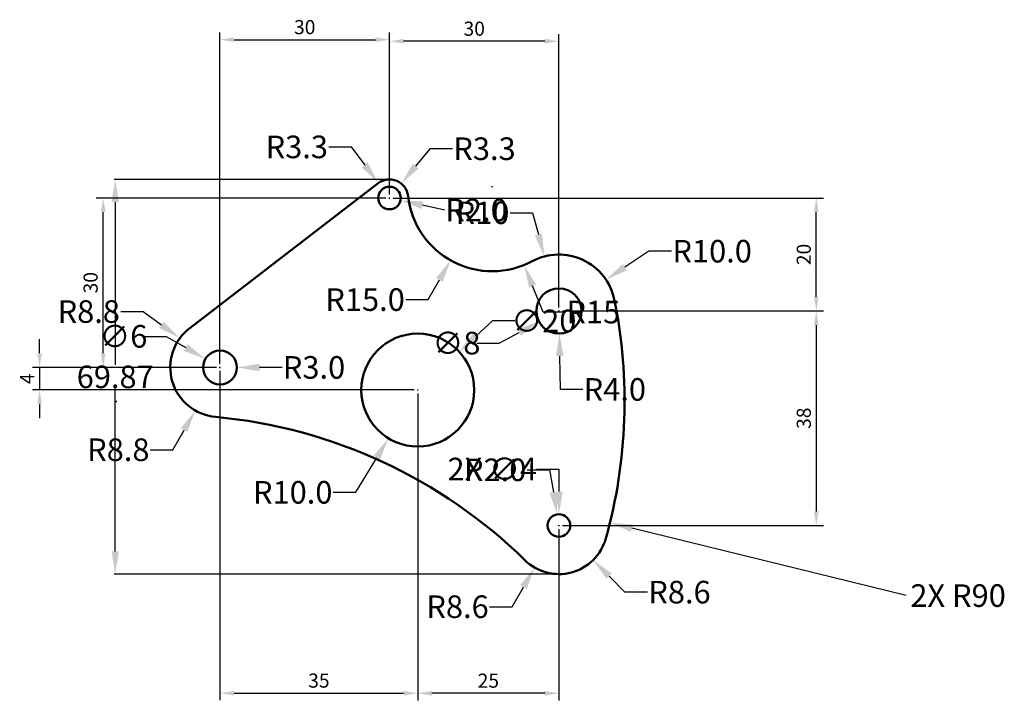
# Model space of a CAD drawing. Units: millimetres. Extents: x 257 to 432, y 502 to 622.
import ezdxf

# ---------------------------------------------------------------- set-up
doc = ezdxf.new("R2010")
doc.units = ezdxf.units.MM
doc.layers.add('M-DIMS', color=2, linetype='Continuous', lineweight=25)
doc.layers.add('M-OUTL', color=7, linetype='Continuous', lineweight=50)
doc.styles.get("Standard").update_dxf_attribs({"font": 'arial.ttf'})
doc.dimstyles.new('ISO-25', dxfattribs={"dimtxt": 2.5, "dimasz": 2.5, "dimexe": 1.25, "dimexo": 0.625, "dimtad": 1, "dimtxsty": 'Standard', "dimcen": 2.5, "dimadec": 0, "dimazin": 0, "dimtfac": 1, "dimtmove": 0, "dimatfit": 3, "dimfxl": 1, "dimarcsym": 0})
doc.dimstyles.get("Standard").update_dxf_attribs({"dimtxt": 4, "dimasz": 4, "dimexe": 0.18, "dimexo": 0.0625, "dimgap": 0.09, "dimtad": 0, "dimtih": 1, "dimtoh": 1, "dimdec": 1, "dimzin": 0, "dimdsep": 46, "dimtxsty": 'Standard', "dimcen": 0.09, "dimadec": 0, "dimazin": 0, "dimtfac": 1, "dimtdec": 1, "dimtofl": 0, "dimtmove": 0, "dimatfit": 3, "dimfxl": 1, "dimtolj": 1, "dimtzin": 0, "dimarcsym": 0})

# ---------------------------------------------------------------- blocks, each defined once
blk = doc.blocks.new('*D1')
at = {"layer": 'Defpoints', "color": 0, "transparency": 16777216}
for p in [(292.89, 560.64), (260.95, 556.64), (327.89, 556.64)]:
    blk.add_point(p, dxfattribs=at)
at = {"layer": 'M-DIMS', "color": 0, "lineweight": -2, "transparency": 16777216}
for p, q in [((260.95, 563.14), (260.95, 565.64)), ((292.27, 560.64), (259.7, 560.64)), ((260.95, 560.64), (260.95, 556.64)), ((327.27, 556.64), (259.7, 556.64)), ((260.95, 554.14), (260.95, 551.64))]:
    blk.add_line(p, q, dxfattribs=at)
at = {"layer": 'M-DIMS', "color": 0, "transparency": 16777216}
for points in [[(260.53, 563.14), (261.36, 563.14), (260.95, 560.64)], [(260.53, 554.14), (261.36, 554.14), (260.95, 556.64)]]:
    blk.add_solid(points, dxfattribs=at)
at = {"layer": 'M-DIMS', "color": 0, "transparency": 16777216, "insert": (259.07, 558.64), "char_height": 2.5, "attachment_point": 5, "rotation": 90}
blk.add_mtext('4', dxfattribs=at)
blk = doc.blocks.new('*D2')
at = {"layer": 'Defpoints', "color": 0, "transparency": 16777216}
for p in [(322.89, 618.4), (322.89, 590.64), (352.89, 570.64)]:
    blk.add_point(p, dxfattribs=at)
at = {"layer": 'M-DIMS', "color": 0, "lineweight": -2, "transparency": 16777216}
for p, q in [((322.89, 591.26), (322.89, 619.65)), ((352.89, 571.26), (352.89, 619.65)), ((350.39, 618.4), (325.39, 618.4))]:
    blk.add_line(p, q, dxfattribs=at)
at = {"layer": 'M-DIMS', "color": 0, "transparency": 16777216}
for points in [[(325.39, 618.82), (325.39, 617.99), (322.89, 618.4)], [(350.39, 618.82), (350.39, 617.99), (352.89, 618.4)]]:
    blk.add_solid(points, dxfattribs=at)
at = {"layer": 'M-DIMS', "color": 0, "transparency": 16777216, "insert": (337.89, 620.3), "char_height": 2.5, "attachment_point": 5}
blk.add_mtext('30', dxfattribs=at)
blk = doc.blocks.new('*D3')
at = {"layer": 'Defpoints', "color": 0, "transparency": 16777216}
for p in [(322.89, 618.68), (322.89, 590.64), (292.89, 560.64)]:
    blk.add_point(p, dxfattribs=at)
at = {"layer": 'M-DIMS', "color": 0, "lineweight": -2, "transparency": 16777216}
for p, q in [((292.89, 561.26), (292.89, 619.93)), ((322.89, 591.26), (322.89, 619.93)), ((295.39, 618.68), (320.39, 618.68))]:
    blk.add_line(p, q, dxfattribs=at)
at = {"layer": 'M-DIMS', "color": 0, "transparency": 16777216}
for points in [[(295.39, 619.09), (295.39, 618.26), (292.89, 618.68)], [(320.39, 619.09), (320.39, 618.26), (322.89, 618.68)]]:
    blk.add_solid(points, dxfattribs=at)
at = {"layer": 'M-DIMS', "color": 0, "transparency": 16777216, "insert": (307.89, 620.58), "char_height": 2.5, "attachment_point": 5}
blk.add_mtext('30', dxfattribs=at)
blk = doc.blocks.new('*D4')
at = {"layer": 'Defpoints', "color": 0, "transparency": 16777216}
for p in [(327.89, 556.64), (352.89, 532.64), (327.89, 502.93)]:
    blk.add_point(p, dxfattribs=at)
at = {"layer": 'M-DIMS', "color": 0, "lineweight": -2, "transparency": 16777216}
for p, q in [((327.89, 556.01), (327.89, 501.68)), ((352.89, 532.01), (352.89, 501.68)), ((350.39, 502.93), (330.39, 502.93))]:
    blk.add_line(p, q, dxfattribs=at)
at = {"layer": 'M-DIMS', "color": 0, "transparency": 16777216}
for points in [[(330.39, 503.35), (330.39, 502.52), (327.89, 502.93)], [(350.39, 503.35), (350.39, 502.52), (352.89, 502.93)]]:
    blk.add_solid(points, dxfattribs=at)
at = {"layer": 'M-DIMS', "color": 0, "transparency": 16777216, "insert": (340.39, 504.84), "char_height": 2.5, "attachment_point": 5}
blk.add_mtext('25', dxfattribs=at)
blk = doc.blocks.new('*D5')
at = {"layer": 'Defpoints', "color": 0, "transparency": 16777216}
for p in [(352.89, 570.64), (352.89, 532.64), (398.45, 532.64)]:
    blk.add_point(p, dxfattribs=at)
at = {"layer": 'M-DIMS', "color": 0, "lineweight": -2, "transparency": 16777216}
for p, q in [((353.52, 570.64), (399.7, 570.64)), ((398.45, 568.14), (398.45, 535.14)), ((353.52, 532.64), (399.7, 532.64))]:
    blk.add_line(p, q, dxfattribs=at)
at = {"layer": 'M-DIMS', "color": 0, "transparency": 16777216}
for points in [[(398.03, 568.14), (398.86, 568.14), (398.45, 570.64)], [(398.03, 535.14), (398.86, 535.14), (398.45, 532.64)]]:
    blk.add_solid(points, dxfattribs=at)
at = {"layer": 'M-DIMS', "color": 0, "transparency": 16777216, "insert": (396.55, 551.64), "char_height": 2.5, "attachment_point": 5, "rotation": 90}
blk.add_mtext('38', dxfattribs=at)
blk = doc.blocks.new('*D6')
at = {"layer": 'Defpoints', "color": 0, "transparency": 16777216}
for p in [(322.89, 590.64), (398.45, 590.64), (352.89, 570.64)]:
    blk.add_point(p, dxfattribs=at)
at = {"layer": 'M-DIMS', "color": 0, "lineweight": -2, "transparency": 16777216}
for p, q in [((323.52, 590.64), (399.7, 590.64)), ((398.45, 573.14), (398.45, 588.14)), ((353.52, 570.64), (399.7, 570.64))]:
    blk.add_line(p, q, dxfattribs=at)
at = {"layer": 'M-DIMS', "color": 0, "transparency": 16777216}
for points in [[(398.03, 588.14), (398.86, 588.14), (398.45, 590.64)], [(398.03, 573.14), (398.86, 573.14), (398.45, 570.64)]]:
    blk.add_solid(points, dxfattribs=at)
at = {"layer": 'M-DIMS', "color": 0, "transparency": 16777216, "insert": (396.55, 580.64), "char_height": 2.5, "attachment_point": 5, "rotation": 90}
blk.add_mtext('20', dxfattribs=at)
blk = doc.blocks.new('*D7')
at = {"layer": 'Defpoints', "color": 0, "transparency": 16777216}
for p in [(292.89, 560.64), (327.89, 556.64), (327.89, 502.94)]:
    blk.add_point(p, dxfattribs=at)
at = {"layer": 'M-DIMS', "color": 0, "lineweight": -2, "transparency": 16777216}
for p, q in [((292.89, 560.01), (292.89, 501.69)), ((327.89, 556.01), (327.89, 501.69)), ((295.39, 502.94), (325.39, 502.94))]:
    blk.add_line(p, q, dxfattribs=at)
at = {"layer": 'M-DIMS', "color": 0, "transparency": 16777216}
for points in [[(295.39, 503.36), (295.39, 502.53), (292.89, 502.94)], [(325.39, 503.36), (325.39, 502.53), (327.89, 502.94)]]:
    blk.add_solid(points, dxfattribs=at)
at = {"layer": 'M-DIMS', "color": 0, "transparency": 16777216, "insert": (310.39, 504.85), "char_height": 2.5, "attachment_point": 5}
blk.add_mtext('35', dxfattribs=at)
blk = doc.blocks.new('*D8')
at = {"layer": 'Defpoints', "color": 0, "transparency": 16777216}
for p in [(272.22, 590.64), (322.89, 590.64), (292.89, 560.64)]:
    blk.add_point(p, dxfattribs=at)
at = {"layer": 'M-DIMS', "color": 0, "lineweight": -2, "transparency": 16777216}
for p, q in [((322.27, 590.64), (270.97, 590.64)), ((272.22, 563.14), (272.22, 588.14)), ((292.27, 560.64), (270.97, 560.64))]:
    blk.add_line(p, q, dxfattribs=at)
at = {"layer": 'M-DIMS', "color": 0, "transparency": 16777216}
for points in [[(271.8, 588.14), (272.63, 588.14), (272.22, 590.64)], [(271.8, 563.14), (272.63, 563.14), (272.22, 560.64)]]:
    blk.add_solid(points, dxfattribs=at)
at = {"layer": 'M-DIMS', "color": 0, "transparency": 16777216, "insert": (270.31, 575.64), "char_height": 2.5, "attachment_point": 5, "rotation": 90}
blk.add_mtext('30', dxfattribs=at)
blk = doc.blocks.new('*D9')
at = {"layer": 'Defpoints', "color": 0, "transparency": 16777216}
for p in [(352.89, 532.64), (358.94, 526.53)]:
    blk.add_point(p, dxfattribs=at)
at = {"layer": 'M-DIMS', "color": 0, "lineweight": -2, "transparency": 16777216}
for p, q in [((352.8, 532.64), (352.98, 532.64)), ((352.89, 532.55), (352.89, 532.73)), ((364.57, 520.84), (361.76, 523.68)), ((368.57, 520.84), (364.57, 520.84))]:
    blk.add_line(p, q, dxfattribs=at)
at = {"layer": 'M-DIMS', "color": 0, "transparency": 16777216}
blk.add_solid([(362.23, 524.15), (361.28, 523.21), (358.94, 526.53)], dxfattribs=at)
at = {"layer": 'M-DIMS', "color": 0, "transparency": 16777216, "insert": (374.22, 520.84), "char_height": 4, "attachment_point": 5}
blk.add_mtext('\\A1;R8.6', dxfattribs=at)
blk = doc.blocks.new('*D10')
at = {"layer": 'Defpoints', "color": 0, "transparency": 16777216}
for p in [(361.22, 576.17), (352.89, 570.64)]:
    blk.add_point(p, dxfattribs=at)
at = {"layer": 'M-DIMS', "color": 0, "lineweight": -2, "transparency": 16777216}
for p, q in [((368.81, 581.22), (364.55, 578.39)), ((372.81, 581.22), (368.81, 581.22)), ((352.8, 570.64), (352.98, 570.64)), ((352.89, 570.55), (352.89, 570.73))]:
    blk.add_line(p, q, dxfattribs=at)
at = {"layer": 'M-DIMS', "color": 0, "transparency": 16777216}
blk.add_solid([(364.18, 578.94), (364.92, 577.83), (361.22, 576.17)], dxfattribs=at)
at = {"layer": 'M-DIMS', "color": 0, "transparency": 16777216, "insert": (380.01, 581.22), "char_height": 4, "attachment_point": 5}
blk.add_mtext('\\A1;R10.0', dxfattribs=at)
blk = doc.blocks.new('*D11')
at = {"layer": 'Defpoints', "color": 0, "transparency": 16777216}
for p in [(292.89, 560.64), (288.52, 553)]:
    blk.add_point(p, dxfattribs=at)
at = {"layer": 'M-DIMS', "color": 0, "lineweight": -2, "transparency": 16777216}
for p, q in [((292.8, 560.64), (292.98, 560.64)), ((292.89, 560.55), (292.89, 560.73)), ((284.54, 546.06), (286.53, 549.53)), ((280.54, 546.06), (284.54, 546.06))]:
    blk.add_line(p, q, dxfattribs=at)
at = {"layer": 'M-DIMS', "color": 0, "transparency": 16777216}
blk.add_solid([(285.95, 549.86), (287.11, 549.2), (288.52, 553)], dxfattribs=at)
at = {"layer": 'M-DIMS', "color": 0, "transparency": 16777216, "insert": (274.89, 546.06), "char_height": 4, "attachment_point": 5}
blk.add_mtext('\\A1;R8.8', dxfattribs=at)
blk = doc.blocks.new('*D12')
at = {"layer": 'Defpoints', "color": 0, "transparency": 16777216}
for p in [(324.98, 593.19), (322.89, 590.64)]:
    blk.add_point(p, dxfattribs=at)
at = {"layer": 'M-DIMS', "color": 0, "lineweight": -2, "transparency": 16777216}
for p, q in [((330.06, 599.37), (327.52, 596.28)), ((334.06, 599.37), (330.06, 599.37)), ((322.8, 590.64), (322.98, 590.64)), ((322.89, 590.55), (322.89, 590.73))]:
    blk.add_line(p, q, dxfattribs=at)
at = {"layer": 'M-DIMS', "color": 0, "transparency": 16777216}
blk.add_solid([(327.01, 596.7), (328.04, 595.85), (324.98, 593.19)], dxfattribs=at)
at = {"layer": 'M-DIMS', "color": 0, "transparency": 16777216, "insert": (339.71, 599.37), "char_height": 4, "attachment_point": 5}
blk.add_mtext('\\A1;R3.3', dxfattribs=at)
blk = doc.blocks.new('*D13')
at = {"layer": 'Defpoints', "color": 0, "transparency": 16777216}
for p in [(341.08, 592.67), (333.7, 579.61)]:
    blk.add_point(p, dxfattribs=at)
at = {"layer": 'M-DIMS', "color": 0, "lineweight": -2, "transparency": 16777216}
for p, q in [((340.99, 592.67), (341.17, 592.67)), ((341.08, 592.58), (341.08, 592.76)), ((329.76, 572.65), (331.73, 576.13)), ((325.76, 572.65), (329.76, 572.65))]:
    blk.add_line(p, q, dxfattribs=at)
at = {"layer": 'M-DIMS', "color": 0, "transparency": 16777216}
blk.add_solid([(331.15, 576.46), (332.31, 575.8), (333.7, 579.61)], dxfattribs=at)
at = {"layer": 'M-DIMS', "color": 0, "transparency": 16777216, "insert": (318.57, 572.65), "char_height": 4, "attachment_point": 5}
blk.add_mtext('\\A1;R15.0', dxfattribs=at)
blk = doc.blocks.new('*D14')
at = {"layer": 'Defpoints', "color": 0, "transparency": 16777216}
for p in [(322.89, 590.64), (324.84, 590.21)]:
    blk.add_point(p, dxfattribs=at)
at = {"layer": 'M-DIMS', "color": 0, "lineweight": -2, "transparency": 16777216}
for p, q in [((322.8, 590.64), (322.98, 590.64)), ((322.89, 590.55), (322.89, 590.73)), ((332.66, 588.51), (328.75, 589.36))]:
    blk.add_line(p, q, dxfattribs=at)
at = {"layer": 'M-DIMS', "color": 0, "transparency": 16777216}
blk.add_solid([(328.9, 590.01), (328.61, 588.71), (324.84, 590.21)], dxfattribs=at)
at = {"layer": 'M-DIMS', "color": 0, "transparency": 16777216, "insert": (338.3, 588.51), "char_height": 4, "attachment_point": 5}
blk.add_mtext('\\A1;R2.0', dxfattribs=at)
blk = doc.blocks.new('*D15')
at = {"layer": 'Defpoints', "color": 0, "transparency": 16777216}
for p in [(327.89, 556.64), (322.72, 548.08)]:
    blk.add_point(p, dxfattribs=at)
at = {"layer": 'M-DIMS', "color": 0, "lineweight": -2, "transparency": 16777216}
for p, q in [((327.8, 556.64), (327.98, 556.64)), ((327.89, 556.55), (327.89, 556.73)), ((316.95, 538.52), (320.65, 544.65)), ((312.95, 538.52), (316.95, 538.52))]:
    blk.add_line(p, q, dxfattribs=at)
at = {"layer": 'M-DIMS', "color": 0, "transparency": 16777216}
blk.add_solid([(320.08, 545), (321.22, 544.31), (322.72, 548.08)], dxfattribs=at)
at = {"layer": 'M-DIMS', "color": 0, "transparency": 16777216, "insert": (305.76, 538.52), "char_height": 4, "attachment_point": 5}
blk.add_mtext('\\A1;R10.0', dxfattribs=at)
blk = doc.blocks.new('*D16')
at = {"layer": 'Defpoints', "color": 0, "transparency": 16777216}
for p in [(352.56, 534.61), (352.89, 532.64)]:
    blk.add_point(p, dxfattribs=at)
at = {"layer": 'M-DIMS', "color": 0, "lineweight": -2, "transparency": 16777216}
for p, q in [((347.24, 542.5), (351.24, 542.5)), ((351.24, 542.5), (351.9, 538.55)), ((352.8, 532.64), (352.98, 532.64)), ((352.89, 532.55), (352.89, 532.73))]:
    blk.add_line(p, q, dxfattribs=at)
at = {"layer": 'M-DIMS', "color": 0, "transparency": 16777216}
blk.add_solid([(352.56, 538.66), (351.24, 538.44), (352.56, 534.61)], dxfattribs=at)
at = {"layer": 'M-DIMS', "color": 0, "transparency": 16777216, "insert": (341.6, 542.5), "char_height": 4, "attachment_point": 5}
blk.add_mtext('\\A1;R2.0', dxfattribs=at)
blk = doc.blocks.new('*D17')
at = {"layer": 'Defpoints', "color": 0, "transparency": 16777216}
for p in [(352.89, 570.64), (352.96, 566.64)]:
    blk.add_point(p, dxfattribs=at)
at = {"layer": 'M-DIMS', "color": 0, "lineweight": -2, "transparency": 16777216}
for p, q in [((352.8, 570.64), (352.98, 570.64)), ((352.89, 570.55), (352.89, 570.73)), ((353.14, 556.74), (353.04, 562.64)), ((357.14, 556.74), (353.14, 556.74))]:
    blk.add_line(p, q, dxfattribs=at)
at = {"layer": 'M-DIMS', "color": 0, "transparency": 16777216}
blk.add_solid([(353.7, 562.65), (352.37, 562.63), (352.96, 566.64)], dxfattribs=at)
at = {"layer": 'M-DIMS', "color": 0, "transparency": 16777216, "insert": (362.78, 556.74), "char_height": 4, "attachment_point": 5}
blk.add_mtext('\\A1;R4.0', dxfattribs=at)
blk = doc.blocks.new('*D18')
at = {"layer": 'Defpoints', "color": 0, "transparency": 16777216}
for p in [(292.89, 560.64), (295.89, 560.64)]:
    blk.add_point(p, dxfattribs=at)
at = {"layer": 'M-DIMS', "color": 0, "lineweight": -2, "transparency": 16777216}
for p, q in [((292.8, 560.64), (292.98, 560.64)), ((292.89, 560.55), (292.89, 560.73)), ((303.89, 560.64), (299.89, 560.64))]:
    blk.add_line(p, q, dxfattribs=at)
at = {"layer": 'M-DIMS', "color": 0, "transparency": 16777216}
blk.add_solid([(299.89, 561.3), (299.89, 559.97), (295.89, 560.64)], dxfattribs=at)
at = {"layer": 'M-DIMS', "color": 0, "transparency": 16777216, "insert": (309.53, 560.64), "char_height": 4, "attachment_point": 5}
blk.add_mtext('\\A1;R3.0', dxfattribs=at)
blk = doc.blocks.new('*D19')
at = {"layer": 'Defpoints', "color": 0, "transparency": 16777216}
for p in [(322.47, 593.91), (274.34, 524.04), (352.89, 524.04)]:
    blk.add_point(p, dxfattribs=at)
at = {"layer": 'M-DIMS', "color": 0, "lineweight": -2, "transparency": 16777216}
for p, q in [((322.41, 593.91), (274.16, 593.91)), ((274.34, 589.91), (274.34, 561.11)), ((274.34, 528.04), (274.34, 556.84)), ((352.82, 524.04), (274.16, 524.04))]:
    blk.add_line(p, q, dxfattribs=at)
at = {"layer": 'M-DIMS', "color": 0, "transparency": 16777216}
for points in [[(273.68, 589.91), (275.01, 589.91), (274.34, 593.91)], [(273.68, 528.04), (275.01, 528.04), (274.34, 524.04)]]:
    blk.add_solid(points, dxfattribs=at)
at = {"layer": 'M-DIMS', "color": 0, "transparency": 16777216, "insert": (274.34, 558.97), "char_height": 4, "attachment_point": 5}
blk.add_mtext('\\A1;69.87', dxfattribs=at)
blk = doc.blocks.new('*D20')
at = {"layer": 'Defpoints', "color": 0, "transparency": 16777216}
for p in [(274.51, 554.61), (361.91, 533.12)]:
    blk.add_point(p, dxfattribs=at)
at = {"layer": 'M-DIMS', "color": 0, "lineweight": -2, "transparency": 16777216}
for p, q in [((274.42, 554.61), (274.6, 554.61)), ((274.51, 554.52), (274.51, 554.7)), ((414.35, 520.23), (365.79, 532.17))]:
    blk.add_line(p, q, dxfattribs=at)
at = {"layer": 'M-DIMS', "color": 0, "transparency": 16777216}
blk.add_solid([(365.95, 532.81), (365.64, 531.52), (361.91, 533.12)], dxfattribs=at)
at = {"layer": 'M-DIMS', "color": 0, "transparency": 16777216, "insert": (423.54, 520.23), "char_height": 4, "attachment_point": 5}
blk.add_mtext('\\A1;2X R90', dxfattribs=at)
blk = doc.blocks.new('*D21')
at = {"layer": 'Defpoints', "color": 0, "transparency": 16777216}
for p in [(341.08, 592.67), (346.71, 578.77)]:
    blk.add_point(p, dxfattribs=at)
at = {"layer": 'M-DIMS', "color": 0, "lineweight": -2, "transparency": 16777216}
for p, q in [((340.99, 592.67), (341.17, 592.67)), ((341.08, 592.58), (341.08, 592.76)), ((350.09, 570.43), (348.22, 575.06)), ((354.09, 570.43), (350.09, 570.43))]:
    blk.add_line(p, q, dxfattribs=at)
at = {"layer": 'M-DIMS', "color": 0, "transparency": 16777216}
blk.add_solid([(348.83, 575.31), (347.6, 574.81), (346.71, 578.77)], dxfattribs=at)
at = {"layer": 'M-DIMS', "color": 0, "transparency": 16777216, "insert": (358.98, 570.43), "char_height": 4, "attachment_point": 5}
blk.add_mtext('\\A1;R15', dxfattribs=at)
blk = doc.blocks.new('*D22')
at = {"layer": 'Defpoints', "color": 0, "transparency": 16777216}
for p in [(350.3, 580.29), (352.89, 570.64)]:
    blk.add_point(p, dxfattribs=at)
at = {"layer": 'M-DIMS', "color": 0, "lineweight": -2, "transparency": 16777216}
for p, q in [((344.23, 588.02), (348.23, 588.02)), ((348.23, 588.02), (349.26, 584.16)), ((352.8, 570.64), (352.98, 570.64)), ((352.89, 570.55), (352.89, 570.73))]:
    blk.add_line(p, q, dxfattribs=at)
at = {"layer": 'M-DIMS', "color": 0, "transparency": 16777216}
blk.add_solid([(349.91, 584.33), (348.62, 583.98), (350.3, 580.29)], dxfattribs=at)
at = {"layer": 'M-DIMS', "color": 0, "transparency": 16777216, "insert": (339.36, 588.02), "char_height": 4, "attachment_point": 5}
blk.add_mtext('\\A1;R10', dxfattribs=at)
blk = doc.blocks.new('*D23')
at = {"layer": 'Defpoints', "color": 0, "transparency": 16777216}
for p in [(285.78, 565.82), (292.89, 560.64)]:
    blk.add_point(p, dxfattribs=at)
at = {"layer": 'M-DIMS', "color": 0, "lineweight": -2, "transparency": 16777216}
for p, q in [((275.31, 570.53), (279.31, 570.53)), ((279.31, 570.53), (282.54, 568.17)), ((292.8, 560.64), (292.98, 560.64)), ((292.89, 560.55), (292.89, 560.73))]:
    blk.add_line(p, q, dxfattribs=at)
at = {"layer": 'M-DIMS', "color": 0, "transparency": 16777216}
blk.add_solid([(282.94, 568.71), (282.15, 567.63), (285.78, 565.82)], dxfattribs=at)
at = {"layer": 'M-DIMS', "color": 0, "transparency": 16777216, "insert": (269.66, 570.53), "char_height": 4, "attachment_point": 5}
blk.add_mtext('\\A1;R8.8', dxfattribs=at)
blk = doc.blocks.new('*D24')
at = {"layer": 'Defpoints', "color": 0, "transparency": 16777216}
for p in [(352.89, 532.64), (348.59, 525.19)]:
    blk.add_point(p, dxfattribs=at)
at = {"layer": 'M-DIMS', "color": 0, "lineweight": -2, "transparency": 16777216}
for p, q in [((352.8, 532.64), (352.98, 532.64)), ((352.89, 532.55), (352.89, 532.73)), ((344.59, 518.26), (346.59, 521.73)), ((340.59, 518.26), (344.59, 518.26))]:
    blk.add_line(p, q, dxfattribs=at)
at = {"layer": 'M-DIMS', "color": 0, "transparency": 16777216}
blk.add_solid([(346.01, 522.06), (347.17, 521.39), (348.59, 525.19)], dxfattribs=at)
at = {"layer": 'M-DIMS', "color": 0, "transparency": 16777216, "insert": (334.94, 518.26), "char_height": 4, "attachment_point": 5}
blk.add_mtext('\\A1;R8.6', dxfattribs=at)
blk = doc.blocks.new('*D25')
at = {"layer": 'Defpoints', "color": 0, "transparency": 16777216}
for p in [(320.92, 593.28), (322.89, 590.64)]:
    blk.add_point(p, dxfattribs=at)
at = {"layer": 'M-DIMS', "color": 0, "lineweight": -2, "transparency": 16777216}
for p, q in [((312.13, 599.69), (316.13, 599.69)), ((316.13, 599.69), (318.52, 596.48)), ((322.8, 590.64), (322.98, 590.64)), ((322.89, 590.55), (322.89, 590.73))]:
    blk.add_line(p, q, dxfattribs=at)
at = {"layer": 'M-DIMS', "color": 0, "transparency": 16777216}
blk.add_solid([(319.05, 596.88), (317.99, 596.08), (320.92, 593.28)], dxfattribs=at)
at = {"layer": 'M-DIMS', "color": 0, "transparency": 16777216, "insert": (306.48, 599.69), "char_height": 4, "attachment_point": 5}
blk.add_mtext('\\A1;R3.3', dxfattribs=at)
blk = doc.blocks.new('*D26')
at = {"layer": 'Defpoints', "color": 0, "transparency": 16777216}
for p in [(335.23, 563.43), (320.55, 549.84)]:
    blk.add_point(p, dxfattribs=at)
at = {"layer": 'M-DIMS', "color": 0, "lineweight": -2, "transparency": 16777216}
for p, q in [((341.1, 568.87), (338.16, 566.15)), ((345.1, 568.87), (341.1, 568.87)), ((327.8, 556.64), (327.98, 556.64)), ((327.89, 556.55), (327.89, 556.73))]:
    blk.add_line(p, q, dxfattribs=at)
at = {"layer": 'M-DIMS', "color": 0, "transparency": 16777216}
blk.add_solid([(337.71, 566.64), (338.61, 565.66), (335.23, 563.43)], dxfattribs=at)
at = {"layer": 'M-DIMS', "color": 0, "transparency": 16777216, "insert": (350.22, 568.87), "char_height": 4, "attachment_point": 5}
blk.add_mtext('\\A1;∅20', dxfattribs=at)
blk = doc.blocks.new('*D27')
at = {"layer": 'Defpoints', "color": 0, "transparency": 16777216}
for p in [(356.41, 572.53), (349.37, 568.74)]:
    blk.add_point(p, dxfattribs=at)
at = {"layer": 'M-DIMS', "color": 0, "lineweight": -2, "transparency": 16777216}
for p, q in [((352.8, 570.64), (352.98, 570.64)), ((352.89, 570.55), (352.89, 570.73)), ((342.33, 564.94), (345.85, 566.84)), ((338.33, 564.94), (342.33, 564.94))]:
    blk.add_line(p, q, dxfattribs=at)
at = {"layer": 'M-DIMS', "color": 0, "transparency": 16777216}
blk.add_solid([(345.53, 567.43), (346.17, 566.25), (349.37, 568.74)], dxfattribs=at)
at = {"layer": 'M-DIMS', "color": 0, "transparency": 16777216, "insert": (334.75, 564.94), "char_height": 4, "attachment_point": 5}
blk.add_mtext('\\A1;∅8', dxfattribs=at)
blk = doc.blocks.new('*D28')
at = {"layer": 'Defpoints', "color": 0, "transparency": 16777216}
for p in [(352.89, 534.64), (352.89, 530.64)]:
    blk.add_point(p, dxfattribs=at)
at = {"layer": 'M-DIMS', "color": 0, "lineweight": -2, "transparency": 16777216}
for p, q in [((348.89, 542.64), (352.89, 542.64)), ((352.89, 542.64), (352.89, 538.64)), ((352.8, 532.64), (352.98, 532.64)), ((352.89, 532.55), (352.89, 532.73))]:
    blk.add_line(p, q, dxfattribs=at)
at = {"layer": 'M-DIMS', "color": 0, "transparency": 16777216}
blk.add_solid([(353.56, 538.64), (352.22, 538.64), (352.89, 534.64)], dxfattribs=at)
at = {"layer": 'M-DIMS', "color": 0, "transparency": 16777216, "insert": (341.09, 542.64), "char_height": 4, "attachment_point": 5}
blk.add_mtext('\\A1;2X ∅4', dxfattribs=at)
blk = doc.blocks.new('*D29')
at = {"layer": 'Defpoints', "color": 0, "transparency": 16777216}
for p in [(290.29, 562.14), (295.49, 559.13)]:
    blk.add_point(p, dxfattribs=at)
at = {"layer": 'M-DIMS', "color": 0, "lineweight": -2, "transparency": 16777216}
for p, q in [((279.37, 566.14), (283.37, 566.14)), ((283.37, 566.14), (286.83, 564.14)), ((292.8, 560.64), (292.98, 560.64)), ((292.89, 560.55), (292.89, 560.73))]:
    blk.add_line(p, q, dxfattribs=at)
at = {"layer": 'M-DIMS', "color": 0, "transparency": 16777216}
blk.add_solid([(287.16, 564.72), (286.5, 563.56), (290.29, 562.14)], dxfattribs=at)
at = {"layer": 'M-DIMS', "color": 0, "transparency": 16777216, "insert": (275.79, 566.14), "char_height": 4, "attachment_point": 5}
blk.add_mtext('\\A1;∅6', dxfattribs=at)

msp = doc.modelspace()

# ---------------------------------------------------------------- linework, layer by layer
at = {"layer": 'M-OUTL'}
msp.add_line((320.879, 593.252), (287.527, 567.613), dxfattribs=at)
for centre, radius in [((322.891, 590.636), 2), ((352.891, 570.636), 4), ((327.891, 556.636), 10), ((292.891, 560.636), 3), ((352.891, 532.636), 2)]:
    msp.add_circle(centre, radius, dxfattribs=at)
for centre, radius, start, end in [((322.891, 590.636), 3.3, 6.37788, 127.55143), ((341.077, 592.669), 15, 186.37788, 298.19868), ((352.891, 570.636), 10, 11.55658, 118.19868), ((274.512, 554.609), 90, 344.33927, 11.55658), ((292.891, 560.636), 8.8, 127.55143, 264.74411), ((283.84, 462.251), 90, 45.54819, 84.74411), ((352.891, 532.636), 8.6, 225.54819, 344.33927)]:
    msp.add_arc(centre, radius, start, end, dxfattribs=at)

# ---------------------------------------------------------------- dimensions: what is measured, and where the dimension line sits
at = {"layer": 'M-DIMS'}
for base, p1, p2, picture, middle in [((322.891, 618.677), (292.891, 560.636), (322.891, 590.636), '*D3', (307.891, 620.579)), ((322.891, 618.402), (352.891, 570.636), (322.891, 590.636), '*D2', (337.891, 620.304)), ((327.891, 502.944), (292.891, 560.636), (327.891, 556.636), '*D7', (310.391, 504.846)), ((327.891, 502.934), (352.891, 532.636), (327.891, 556.636), '*D4', (340.391, 504.836))]:
    dim = msp.add_linear_dim(base=base, p1=p1, p2=p2, dimstyle='ISO-25', override={"dimclrd": 0, "dimclre": 0, "dimclrt": 0}, dxfattribs=at)
    dim.commit()
    dim.dimension.update_dxf_attribs({"geometry": picture, "text_midpoint": middle})
for center, mpoint, override, picture, middle in [((322.891, 590.636), (320.915, 593.28), {"dimdec": 1, "dimlfac": 1, "dimrnd": 0, "dimzin": 0, "dimdsep": 46, "dimlunit": 2}, '*D25', (306.481, 599.688)), ((322.891, 590.636), (324.985, 593.186), {"dimclrd": 0, "dimclre": 0, "dimclrt": 0}, '*D12', (339.707, 599.369)), ((341.077, 592.669), (333.696, 579.611), {"dimclrd": 0, "dimclre": 0, "dimclrt": 0}, '*D13', (318.567, 572.646)), ((322.891, 590.636), (324.845, 590.211), {"dimclrd": 0, "dimclre": 0, "dimclrt": 0}, '*D14', (338.301, 588.511)), ((352.891, 570.636), (350.299, 580.294), {"dimdec": 0, "dimlfac": 1, "dimrnd": 0, "dimzin": 0, "dimdsep": 46, "dimlunit": 2}, '*D22', (339.363, 588.021)), ((292.891, 560.636), (285.777, 565.817), {"dimdec": 1, "dimlfac": 1, "dimrnd": 0, "dimzin": 0, "dimdsep": 46, "dimlunit": 2}, '*D23', (269.661, 570.526)), ((292.891, 560.636), (295.891, 560.636), {"dimclrd": 0, "dimclre": 0, "dimclrt": 0}, '*D18', (309.529, 560.636)), ((292.891, 560.636), (288.518, 552.999), {"dimclrd": 0, "dimclre": 0, "dimclrt": 0}, '*D11', (274.893, 546.057)), ((352.891, 532.636), (352.561, 534.609), {"dimclrd": 0, "dimclre": 0, "dimclrt": 0}, '*D16', (341.605, 542.499)), ((352.891, 532.636), (348.589, 525.189), {"dimdec": 1, "dimlfac": 1, "dimrnd": 0, "dimzin": 0, "dimdsep": 46, "dimlunit": 2}, '*D24', (334.944, 518.261)), ((352.891, 532.636), (358.942, 526.525), {"dimclrd": 0, "dimclre": 0, "dimclrt": 0}, '*D9', (374.215, 520.841))]:
    dim = msp.add_radius_dim(center=center, mpoint=mpoint, dimstyle='Standard', override=override, dxfattribs=at)
    dim.commit()
    dim.dimension.update_dxf_attribs({"geometry": picture, "text_midpoint": middle})
for base, p1, p2, dimstyle, override, picture, middle in [((274.342, 524.036), (322.474, 593.91), (352.887, 524.036), 'Standard', {"dimdec": 2, "dimlfac": 1, "dimrnd": 0, "dimzin": 0, "dimdsep": 46, "dimlunit": 2}, '*D19', (274.342, 558.973)), ((272.216, 590.636), (292.891, 560.636), (322.891, 590.636), 'ISO-25', {"dimclrd": 0, "dimclre": 0, "dimclrt": 0}, '*D8', (270.314, 575.636)), ((398.448, 590.636), (352.891, 570.636), (322.891, 590.636), 'ISO-25', {"dimclrd": 0, "dimclre": 0, "dimclrt": 0}, '*D6', (396.547, 580.636)), ((398.448, 532.636), (352.891, 570.636), (352.891, 532.636), 'ISO-25', {"dimclrd": 0, "dimclre": 0, "dimclrt": 0}, '*D5', (396.546, 551.636)), ((260.948, 556.636), (292.891, 560.636), (327.891, 556.636), 'ISO-25', {"dimclrd": 0, "dimclre": 0, "dimclrt": 0}, '*D1', (259.073, 558.636))]:
    dim = msp.add_linear_dim(base=base, p1=p1, p2=p2, angle=90, dimstyle=dimstyle, override=override, dxfattribs=at)
    dim.commit()
    dim.dimension.update_dxf_attribs({"geometry": picture, "text_midpoint": middle})
for center, mpoint, override, picture, middle in [((341.077, 592.669), (346.713, 578.768), {"dimdec": 0, "dimlfac": 1, "dimrnd": 0, "dimzin": 0, "dimdsep": 46, "dimlunit": 2}, '*D21', (358.978, 570.427)), ((352.891, 570.636), (361.219, 576.172), {"dimclrd": 0, "dimclre": 0, "dimclrt": 0}, '*D10', (380.006, 581.221)), ((352.891, 570.636), (352.963, 566.637), {"dimclrd": 0, "dimclre": 0, "dimclrt": 0}, '*D17', (362.78, 556.741)), ((327.891, 556.636), (322.721, 548.076), {"dimclrd": 0, "dimclre": 0, "dimclrt": 0}, '*D15', (305.761, 538.524))]:
    dim = msp.add_radius_dim(center=center, mpoint=mpoint, dimstyle='Standard', override=override, dxfattribs=at)
    dim.commit()
    dim.dimension.update_dxf_attribs({"geometry": picture, "text_midpoint": middle, "dimtype": 164})
for p1, p2, picture, middle in [((356.411, 572.535), (349.37, 568.738), '*D27', (334.747, 564.941)), ((320.555, 549.84), (335.227, 563.432), '*D26', (350.219, 568.869)), ((295.488, 559.134), (290.294, 562.138), '*D29', (275.793, 566.143))]:
    dim = msp.add_diameter_dim_2p(p1=p1, p2=p2, dimstyle='Standard', override={"dimdec": 0, "dimlfac": 1, "dimrnd": 0, "dimzin": 0, "dimdsep": 46, "dimlunit": 2}, dxfattribs=at)
    dim.commit()
    dim.dimension.update_dxf_attribs({"geometry": picture, "text_midpoint": middle, "dimtype": 163})
dim = msp.add_radius_dim(center=(274.512, 554.609), mpoint=(361.91, 533.122), text='2X <>', dimstyle='Standard', override={"dimdec": 0, "dimlfac": 1, "dimrnd": 0, "dimzin": 0, "dimdsep": 46, "dimlunit": 2}, dxfattribs=at)
dim.commit()
dim.dimension.update_dxf_attribs({"geometry": '*D20', "text_midpoint": (414.348, 520.23), "dimtype": 164})
dim = msp.add_diameter_dim_2p(p1=(352.891, 530.636), p2=(352.89, 534.636), text='2X <>', dimstyle='Standard', override={"dimdec": 0, "dimlfac": 1, "dimrnd": 0, "dimzin": 0, "dimdsep": 46, "dimlunit": 2}, dxfattribs=at)
dim.commit()
dim.dimension.update_dxf_attribs({"geometry": '*D28', "text_midpoint": (341.093, 542.636), "dimtype": 163})

doc.saveas('drawing.dxf')
